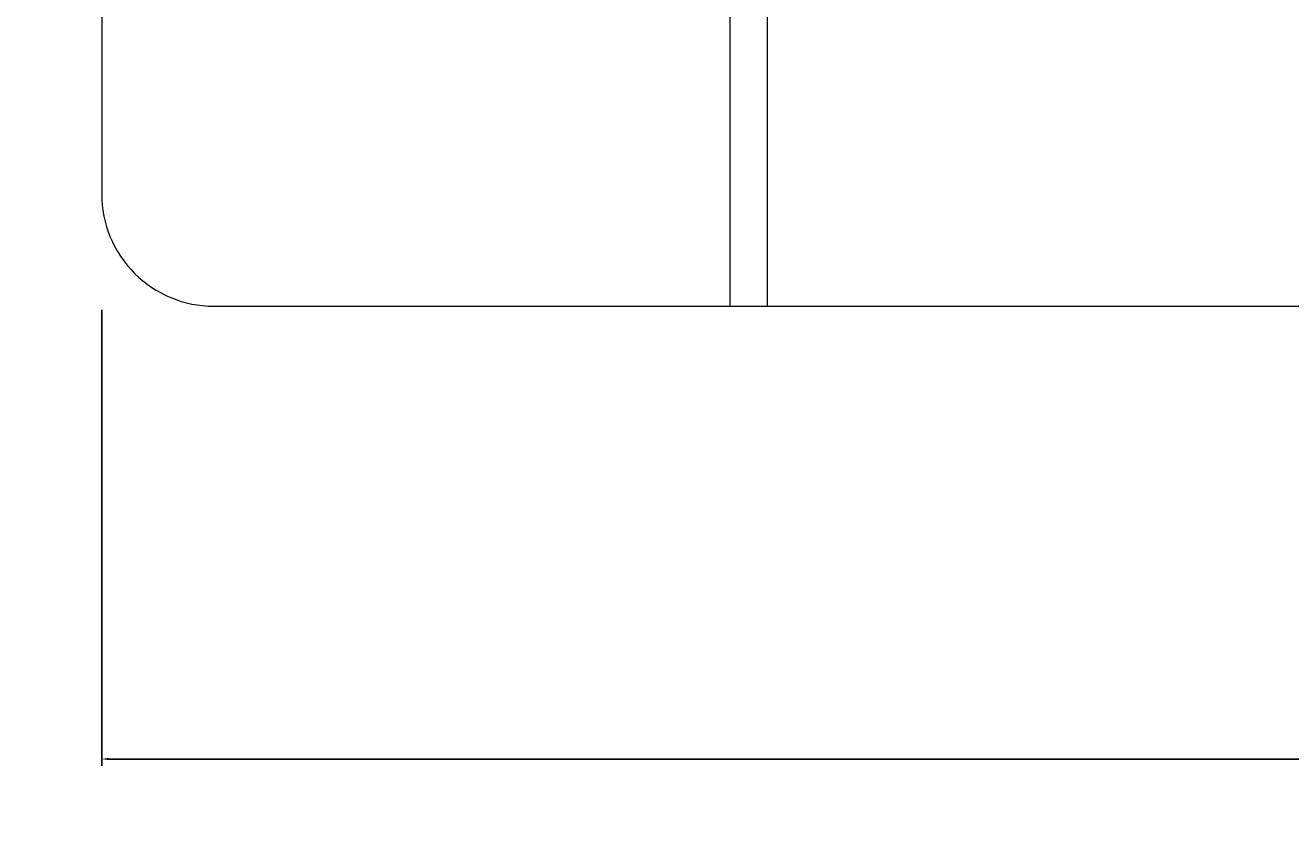
# Model space of a CAD drawing. Units: inches. Extents: x -61 to 1599, y -1316 to 257.
# Tile 146 of 204: x 406 to 440, y 52 to 74. Entities that reach past the tile are written whole.
import ezdxf

# ---------------------------------------------------------------- set-up
doc = ezdxf.new("R2010")
doc.units = ezdxf.units.IN
doc.header["$MEASUREMENT"] = 0
doc.layers.add('A-ANNO-DIMS', color=2, linetype='Continuous', lineweight=18)
doc.layers.add('FURNITURE', color=83, linetype='Continuous', lineweight=18)
doc.styles.get("Standard").update_dxf_attribs({"font": 'arial.ttf'})
doc.dimstyles.get("Standard").update_dxf_attribs({"dimtxt": 0.18, "dimasz": 0.18, "dimexe": 0.18, "dimexo": 0.0625, "dimgap": 0.09, "dimtad": 0, "dimtih": 1, "dimtoh": 1, "dimdec": 0, "dimzin": 0, "dimdsep": 46, "dimlunit": 3, "dimtxsty": 'Standard', "dimcen": 0.09, "dimadec": 0, "dimazin": 0, "dimtfac": 1, "dimtdec": 0, "dimtofl": 0, "dimtmove": 0, "dimatfit": 3, "dimfxl": 1, "dimtolj": 1, "dimtzin": 0, "dimarcsym": 0})

# ---------------------------------------------------------------- blocks, each defined once
blk = doc.blocks.new('BED-DOUBLE-COMPACT')
for p, q in [((16.8, 60.036), (16.8, 0.036)), ((17.8, 60.036), (17.8, 0.036))]:
    blk.add_line(p, q)
blk.add_lwpolyline([(77, 60.036), (3, 60.036, 0.414214), (0, 57.036), (0, 3.036, 0.414214), (3, 0.036), (77, 0.036, 0.414214), (80, 3.036), (80, 57.036, 0.414214)], format="xyb", close=True)
blk = doc.blocks.new('*D676')
at = {"layer": 'A-ANNO-DIMS', "color": 0, "lineweight": -2, "transparency": 16777216}
for p, q in [((407.794, 66.667), (407.794, 54.467)), ((488.345, 66.667), (488.345, 54.467)), ((407.974, 54.647), (446.586, 54.647)), ((488.165, 54.647), (449.554, 54.647))]:
    blk.add_line(p, q, dxfattribs=at)
at = {"layer": 'A-ANNO-DIMS', "color": 0, "transparency": 16777216}
for points in [[(407.974, 54.677), (407.974, 54.617), (407.794, 54.647)], [(488.165, 54.677), (488.165, 54.617), (488.345, 54.647)]]:
    blk.add_solid(points, dxfattribs=at)
at = {"layer": 'DEFPOINTS', "color": 0, "transparency": 16777216}
for p in [(407.794, 66.729), (488.345, 66.729), (488.345, 54.647)]:
    blk.add_point(p, dxfattribs=at)
at = {"layer": 'A-ANNO-DIMS', "color": 0, "transparency": 16777216, "insert": (448.07, 54.647), "char_height": 0.18, "attachment_point": 5}
blk.add_mtext('\\A1;COMPACT BED 81 TYP.', dxfattribs=at)
blk = doc.blocks.new('*D703')
at = {"layer": 'A-ANNO-DIMS', "color": 0, "lineweight": -2, "transparency": 16777216}
for p, q in [((372.32, -616.882), (372.32, 257.457)), ((455.833, -616.882), (455.833, 257.457)), ((372.5, 257.277), (413.7, 257.277)), ((455.653, 257.277), (414.453, 257.277))]:
    blk.add_line(p, q, dxfattribs=at)
at = {"layer": 'A-ANNO-DIMS', "color": 0, "transparency": 16777216}
for points in [[(372.5, 257.307), (372.5, 257.247), (372.32, 257.277)], [(455.653, 257.307), (455.653, 257.247), (455.833, 257.277)]]:
    blk.add_solid(points, dxfattribs=at)
at = {"layer": 'DEFPOINTS', "color": 0, "transparency": 16777216}
for p in [(455.833, 257.277), (372.32, -616.945), (455.833, -616.945)]:
    blk.add_point(p, dxfattribs=at)
at = {"layer": 'A-ANNO-DIMS', "color": 0, "transparency": 16777216, "insert": (414.076, 257.277), "char_height": 0.18, "attachment_point": 5}
blk.add_mtext('\\A1;83.51', dxfattribs=at)

msp = doc.modelspace()

# ---------------------------------------------------------------- block references
at = {"layer": 'FURNITURE'}
msp.add_blockref('BED-DOUBLE-COMPACT', (407.794, 66.733), dxfattribs=at)

# ---------------------------------------------------------------- dimensions: what is measured, and where the dimension line sits
at = {"layer": 'A-ANNO-DIMS'}
dim = msp.add_linear_dim(base=(455.8327, 257.2771), p1=(372.3201, -616.9446), p2=(455.8327, -616.9446), dimstyle='Standard', override={"dimdec": 2, "dimlfac": 1, "dimrnd": 0, "dimzin": 0, "dimdsep": 46, "dimlunit": 2}, dxfattribs=at)
dim.commit()
dim.dimension.update_dxf_attribs({"geometry": '*D703', "text_midpoint": (414.0764, 257.2771)})
dim = msp.add_linear_dim(base=(488.3448, 54.6469), p1=(407.7945, 66.7295), p2=(488.3448, 66.7295), text='COMPACT BED <> TYP.', dimstyle='Standard', override={"dimdec": 0, "dimlfac": 1, "dimrnd": 0, "dimzin": 0, "dimdsep": 46, "dimlunit": 2}, dxfattribs=at)
dim.commit()
dim.dimension.update_dxf_attribs({"geometry": '*D676', "text_midpoint": (448.0696, 54.6469)})

doc.saveas('drawing.dxf')
